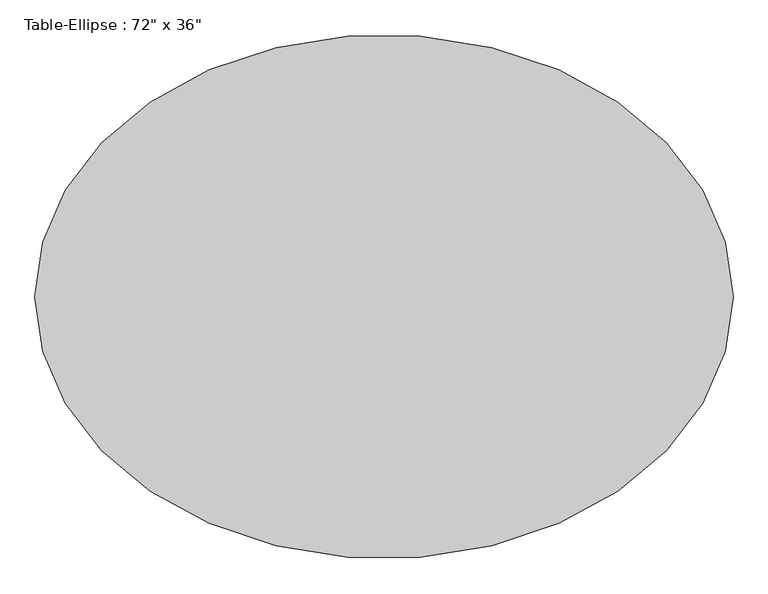
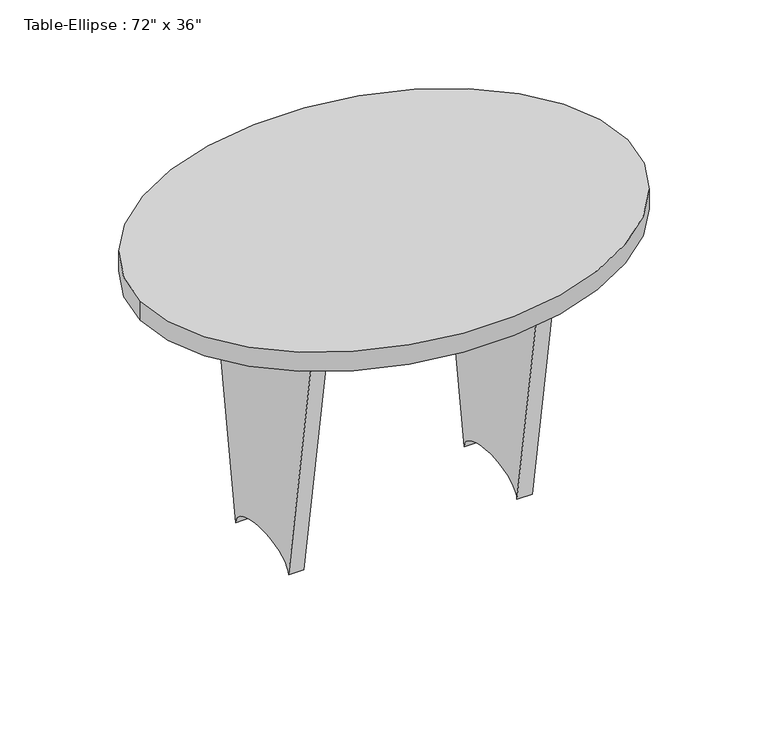
"""IFC4 building model written with IfcOpenShell, lengths in millimetres: furniture geometry."""

from ifc_helpers import new_model, si_unit, point, frame, origin, place, context, project, spatial, ellipse_curve, trimmed, source, transform, mapped, element, save
from ifc_brep_helpers import plane_surface, extruded_surface, advanced_brep


def furniture_cd2394ed(model_context):
    return source(origin(), model_context, "Body", "AdvancedBrep", [
        advanced_brep(
        [(-266.7, 19.05, 711.2), (266.7, 19.05, 711.2), (266.7, 19.05, 474.1333333), (-266.7, 19.05, 474.1333333), (-266.7, -19.05, 711.2), (-266.7, -19.05, 474.1333333), (266.7, -19.05, 474.1333333), (266.7, -19.05, 711.2)],
        [
            (0, 1),
            (1, 2),
            (2, 3, ellipse_curve(frame((0.0, 19.05, 474.1333333), z_axis=(0.0, -1.0, 0.0), x_axis=(1.0, 0.0, 0.0)), 266.7, 101.6)),
            (3, 0),
            (4, 5),
            (5, 6, ellipse_curve(frame((0.0, -19.05, 474.1333333), z_axis=(0.0, 1.0, 0.0), x_axis=(1.0, 0.0, 0.0)), 266.7, 101.6)),
            (6, 7),
            (7, 4),
            (0, 4),
            (7, 1),
            (6, 2),
            (5, 3),
        ],
        [
            plane_surface(frame((-266.7, 19.05, 711.2), z_axis=(0.0, 1.0, 0.0), x_axis=(1.0, 0.0, 0.0))),
            plane_surface(frame((-266.7, -19.05, 711.2), z_axis=(0.0, -1.0, 0.0), x_axis=(-1.0, 0.0, 0.0))),
            plane_surface(frame((-266.7, 19.05, 711.2), z_axis=(0.0, 0.0, 1.0), x_axis=(0.0, -1.0, 0.0))),
            plane_surface(frame((266.7, 19.05, 711.2), z_axis=(1.0, 0.0, 0.0), x_axis=(0.0, -1.0, 0.0))),
            extruded_surface(trimmed(ellipse_curve(frame((0.0, -57.15, 474.1333333), z_axis=(0.0, -1.0, 0.0), x_axis=(1.0, 0.0, 0.0)), 266.7, 101.6), [point((266.7, -57.15, 474.1333333))], [point((-266.7, -57.15, 474.1333333))], True, "CARTESIAN"), (0.0, 38.099999999999994, 0.0), 38.099999999999994),
            plane_surface(frame((-266.7, 19.05, 474.1333333), z_axis=(-1.0, 0.0, 0.0), x_axis=(0.0, -1.0, 0.0))),
        ],
        [
            (0, [[1, 2, 3, 4]]),
            (1, [[5, 6, 7, 8]]),
            (2, [[-1, 9, -8, 10]]),
            (3, [[-2, -10, -7, 11]]),
            (4, [[-3, -11, -6, 12]]),
            (5, [[-4, -12, -5, -9]]),
        ],
    ),
        advanced_brep(
        [(304.8, 228.6, 711.2), (304.8, -228.6, 711.2), (304.8, -114.3, 0.0), (304.8, 114.3, 0.0), (266.7, 228.6, 711.2), (266.7, 114.3, 0.0), (266.7, -114.3, 0.0), (266.7, -228.6, 711.2)],
        [
            (0, 1),
            (1, 2),
            (2, 3, ellipse_curve(frame((304.8, 0.0, 0.0), z_axis=(-1.0, 0.0, 0.0), x_axis=(0.0, 1.0, 0.0)), 114.3, 50.8)),
            (3, 0),
            (4, 5),
            (5, 6, ellipse_curve(frame((266.7, 0.0, 0.0), z_axis=(1.0, 0.0, 0.0), x_axis=(0.0, 1.0, 0.0)), 114.3, 50.8)),
            (6, 7),
            (7, 4),
            (0, 4),
            (7, 1),
            (6, 2),
            (5, 3),
        ],
        [
            plane_surface(frame((304.8, -228.6, 711.2), z_axis=(1.0, 0.0, 0.0), x_axis=(0.0, -1.0, 0.0))),
            plane_surface(frame((266.7, -228.6, 711.2), z_axis=(-1.0, 0.0, 0.0), x_axis=(0.0, 1.0, 0.0))),
            plane_surface(frame((304.8, 228.6, 711.2), z_axis=(0.0, 0.0, 1.0), x_axis=(-1.0, 0.0, 0.0))),
            plane_surface(frame((304.8, -228.6, 711.2), z_axis=(0.0, -0.9873303712766982, -0.158678095383759), x_axis=(-1.0, 0.0, 0.0))),
            extruded_surface(trimmed(ellipse_curve(frame((228.6, 0.0, 0.0), z_axis=(-1.0, 0.0, 0.0), x_axis=(0.0, 1.0, 0.0)), 114.3, 50.8), [point((228.6, -114.3, 0.0))], [point((228.6, 114.3, 0.0))], True, "CARTESIAN"), (38.099999999999994, 0.0, 0.0), 38.099999999999994),
            plane_surface(frame((304.8, 114.3, 0.0), z_axis=(0.0, 0.9873303712767002, -0.15867809538374666), x_axis=(-1.0, 0.0, 0.0))),
        ],
        [
            (0, [[1, 2, 3, 4]]),
            (1, [[5, 6, 7, 8]]),
            (2, [[-1, 9, -8, 10]]),
            (3, [[-2, -10, -7, 11]]),
            (4, [[-3, -11, -6, 12]]),
            (5, [[-4, -12, -5, -9]]),
        ],
    ),
        advanced_brep(
        [(-266.7, 228.6, 711.2), (-266.7, -228.6, 711.2), (-266.7, -114.3, 0.0), (-266.7, 114.3, 0.0), (-304.8, 228.6, 711.2), (-304.8, 114.3, 0.0), (-304.8, -114.3, 0.0), (-304.8, -228.6, 711.2)],
        [
            (0, 1),
            (1, 2),
            (2, 3, ellipse_curve(frame((-266.7, 0.0, 0.0), z_axis=(-1.0, 0.0, 0.0), x_axis=(0.0, 1.0, 0.0)), 114.3, 50.8)),
            (3, 0),
            (4, 5),
            (5, 6, ellipse_curve(frame((-304.8, 0.0, 0.0), z_axis=(1.0, 0.0, 0.0), x_axis=(0.0, 1.0, 0.0)), 114.3, 50.8)),
            (6, 7),
            (7, 4),
            (0, 4),
            (7, 1),
            (6, 2),
            (5, 3),
        ],
        [
            plane_surface(frame((-266.7, -228.6, 711.2), z_axis=(1.0, 0.0, 0.0), x_axis=(0.0, -1.0, 0.0))),
            plane_surface(frame((-304.8, -228.6, 711.2), z_axis=(-1.0, 0.0, 0.0), x_axis=(0.0, 1.0, 0.0))),
            plane_surface(frame((-266.7, 228.6, 711.2), z_axis=(0.0, 0.0, 1.0), x_axis=(-1.0, 0.0, 0.0))),
            plane_surface(frame((-266.7, -228.6, 711.2), z_axis=(0.0, -0.9873303712766983, -0.15867809538375854), x_axis=(-1.0, 0.0, 0.0))),
            extruded_surface(trimmed(ellipse_curve(frame((-342.9, 0.0, 0.0), z_axis=(-1.0, 0.0, 0.0), x_axis=(0.0, 1.0, 0.0)), 114.3, 50.8), [point((-342.9, -114.3, 0.0))], [point((-342.9, 114.3, 0.0))], True, "CARTESIAN"), (38.099999999999966, 0.0, 0.0), 38.099999999999966),
            plane_surface(frame((-266.7, 114.3, 0.0), z_axis=(0.0, 0.9873303712766998, -0.15867809538374977), x_axis=(-1.0, 0.0, 0.0))),
        ],
        [
            (0, [[1, 2, 3, 4]]),
            (1, [[5, 6, 7, 8]]),
            (2, [[-1, 9, -8, 10]]),
            (3, [[-2, -10, -7, 11]]),
            (4, [[-3, -11, -6, 12]]),
            (5, [[-4, -12, -5, -9]]),
        ],
    ),
        advanced_brep(
        [(-609.6, 0.0, 762.0), (609.6, 0.0, 762.0), (-609.6, 0.0, 711.2), (609.6, 0.0, 711.2)],
        [
            (0, 1, ellipse_curve(frame((0.0, 0.0, 762.0), z_axis=(0.0, 0.0, 1.0), x_axis=(1.0, 0.0, 0.0)), 609.6, 457.2)),
            (1, 0, ellipse_curve(frame((0.0, 0.0, 762.0), z_axis=(0.0, 0.0, 1.0), x_axis=(1.0, 0.0, 0.0)), 609.6, 457.2)),
            (2, 3, ellipse_curve(frame((0.0, 0.0, 711.2), z_axis=(0.0, 0.0, -1.0), x_axis=(1.0, 0.0, 0.0)), 609.6, 457.2)),
            (3, 2, ellipse_curve(frame((0.0, 0.0, 711.2), z_axis=(0.0, 0.0, -1.0), x_axis=(1.0, 0.0, 0.0)), 609.6, 457.2)),
            (0, 2),
            (3, 1),
        ],
        [
            plane_surface(frame((609.6, 0.0, 762.0), z_axis=(0.0, 0.0, 1.0), x_axis=(0.0, 1.0, 0.0))),
            plane_surface(frame((609.6, 0.0, 711.2), z_axis=(0.0, 0.0, -1.0), x_axis=(0.0, -1.0, 0.0))),
            extruded_surface(trimmed(ellipse_curve(frame((0.0, 0.0, 660.4), z_axis=(0.0, 0.0, 1.0), x_axis=(1.0, 0.0, 0.0)), 609.6, 457.2), [point((-609.6, 0.0, 660.4))], [point((609.6, 0.0, 660.4))], True, "CARTESIAN"), (0.0, 0.0, 50.80000000000007), 50.80000000000007),
            extruded_surface(trimmed(ellipse_curve(frame((0.0, 0.0, 660.4), z_axis=(0.0, 0.0, 1.0), x_axis=(1.0, 0.0, 0.0)), 609.6, 457.2), [point((609.6, 0.0, 660.4))], [point((-609.6, 0.0, 660.4))], True, "CARTESIAN"), (0.0, 0.0, 50.80000000000007), 50.80000000000007),
        ],
        [
            (0, [[1, 2]]),
            (1, [[3, 4]]),
            (2, [[-1, 5, -4, 6]]),
            (3, [[-2, -6, -3, -5]]),
        ],
    ),
    ])


if __name__ == "__main__":
    model = new_model("IFC4")
    model_context = context("Model", 3, world=origin())
    ifc_project = project(units=[si_unit("LENGTHUNIT", "METRE", prefix="MILLI")], contexts=[model_context])
    site = spatial("IfcSite", under=ifc_project)
    building = spatial("IfcBuilding", under=site)
    placement = place(None, origin())
    furniture_shape = furniture_cd2394ed(model_context)
    element("IfcFurniture", 1, ObjectType="Table-Ellipse : 72\" x 36\"", at=placement, inside=building, context=model_context, shape_type="MappedRepresentation", body=[
        mapped(furniture_shape, transform((0.0, 0.0, 0.0), x_axis=(1.0, 0.0, 0.0), y_axis=(0.0, 1.0, 0.0), z_axis=(0.0, 0.0, 1.0))),
    ])
    save(model, "model.ifc")

# Revit data of these elements
# Type "Table-Ellipse : 72\" x 36\""
#   Assembly Code = "E2020200"
#   Half Width = 1' - 6"
#   Half Length = 2' - 0"
#   Height = 2' - 6"
#   Length = 4' - 0"
#   Width = 3' - 0"
#   Base Material = Birch
#   Top Material = Laminate - Black
#   Default Elevation = 0
# Element 1 (IfcFurniture, "Table-Ellipse : 72\" x 36\"")
#   Materials on its faces: "Birch", "Laminate - Black"
# Materials
#   "Birch": class "Wood", colour RGB 224 178 126, transparency 0, Description = "Betula Alleghaniensis", Cost = 0
#   "Laminate - Black": colour RGB 0 0 0, transparency 0
